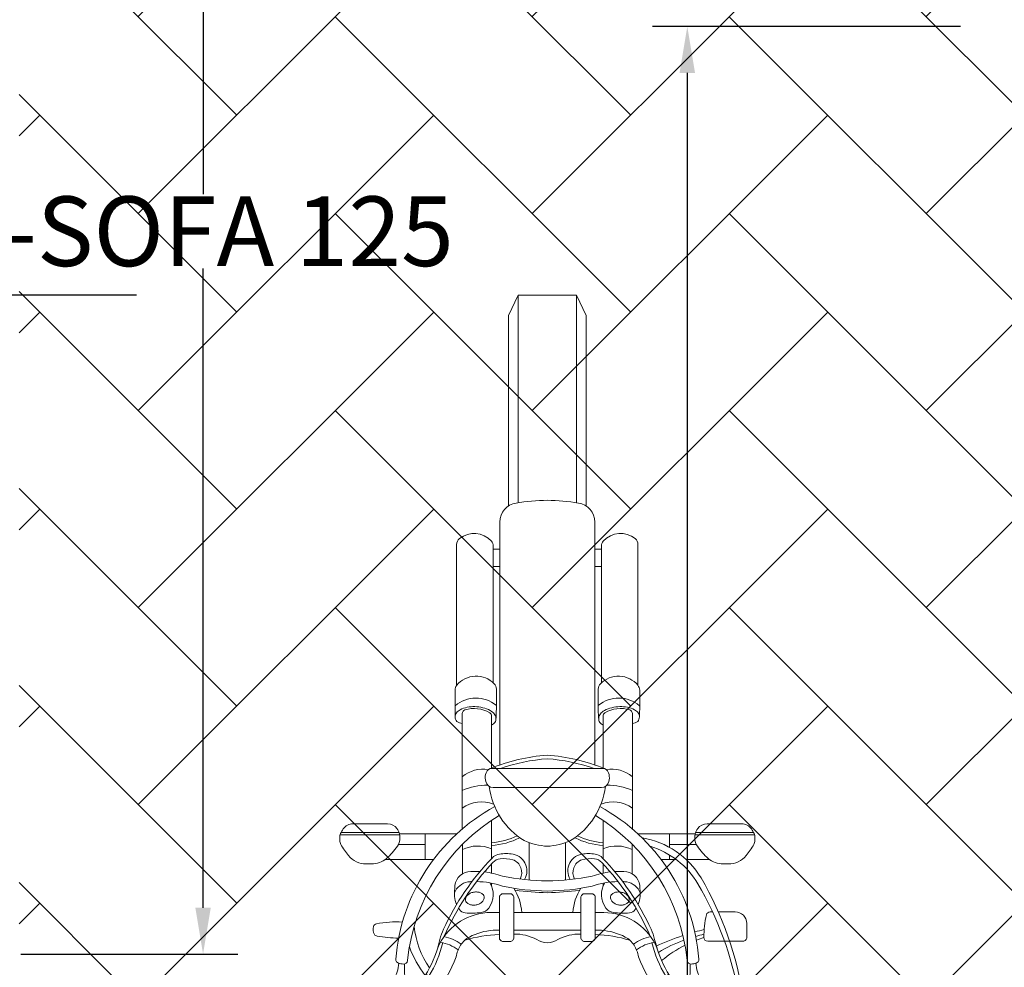
# Model space of a CAD drawing. Units: inches. Extents: x -466983 to 1020, y 324 to 318697.
# Tile 25 of 97: x 814 to 899, y 511 to 592. Entities that reach past the tile are written whole.
import ezdxf

# ---------------------------------------------------------------- set-up
doc = ezdxf.new("R2010")
doc.units = ezdxf.units.IN
doc.header["$MEASUREMENT"] = 0
for name, color, linetype, lineweight in [('A-ANNO-DIMS', 2, 'Continuous', 18), ('A-EQPM-VEHC', 8, 'Continuous', 18), ('A-FLOR-PATT', 252, 'Continuous', 13)]:
    doc.layers.add(name, color=color, linetype=linetype, lineweight=lineweight)
doc.styles.get("Standard").update_dxf_attribs({"font": 'arial.ttf'})
doc.dimstyles.get("Standard").update_dxf_attribs({"dimtxt": 6, "dimasz": 4, "dimexe": 3, "dimexo": 3, "dimgap": 0.09, "dimtad": 0, "dimtih": 1, "dimtoh": 1, "dimdec": 1, "dimzin": 0, "dimdsep": 46, "dimlunit": 3, "dimtxsty": 'Standard', "dimcen": 0.09, "dimadec": 0, "dimazin": 0, "dimtfac": 1, "dimtdec": 1, "dimtofl": 0, "dimtmove": 0, "dimatfit": 3, "dimfxl": 1, "dimtolj": 1, "dimtzin": 0, "dimarcsym": 0})

# ---------------------------------------------------------------- blocks, each defined once
blk = doc.blocks.new('Bike')
for p, q in [((3716.6, 1477), (3739.4, 1477)), ((3715.3, 1469.7), (3739.4, 1469.7)), ((3715, 1462.6), (3739.4, 1462.6)), ((3725.9, 1437.8), (3739.4, 1455.6)), ((3476.2, 1372.3), (3476.2, 1447.6)), ((3479.4, 1371.4), (3479.4, 1449.1)), ((3739.4, 1429.3), (3753.1, 1429.3)), ((4796.8, 1363.8), (4796.8, 1434.1)), ((3739.4, 1420.3), (3753.1, 1420.3)), ((3739.4, 1414.7), (3753.1, 1414.7)), ((3668.6, 1399.5), (3702.1, 1372.5)), ((3671.4, 1403.4), (3705.4, 1376.1)), ((3511.5, 1359.9), (3511.5, 1390.3)), ((4502.2, 1381), (4505.8, 1282.1)), ((3478.1, 1297.1), (3478.1, 1372)), ((3491.8, 1338.1), (3491.8, 1373.1)), ((4781.5, 1364.7), (4781.5, 1326.4)), ((3478.1, 1338.1), (3495.7, 1338.1)), ((3505.6, 1338.1), (3511.5, 1338.1)), ((3511.5, 1346.8), (3511.5, 1327.3)), ((4762.6, 1326.4), (4793.8, 1326.4)), ((4035.1, 1288.5), (4035.1, 1302.5)), ((3491.8, 1289.6), (3530.3, 1289.6)), ((4012.9, 1254.3), (4013.4, 1288.4)), ((4721.1, 1279.7), (4737.7, 1247.6)), ((4738.5, 1279.5), (4753.4, 1246.1)), ((3106.7, 1249.4), (3106.7, 1240.7)), ((3129.5, 1249.4), (3129.5, 1240.7)), ((3460.4, 1251.7), (3510.3, 1251.7)), ((3517.1, 1251.6), (3529.2, 1251.6)), ((3542.4, 1251.6), (3546.2, 1251.6)), ((4896.6, 1245.7), (4912.2, 1245.7)), ((3808.6, 1222.8), (3886.6, 1138)), ((3808.6, 1134.7), (3886.6, 1219.4)), ((3489.4, 1202.6), (3538.3, 1202.6)), ((3489.4, 1155.3), (3538.3, 1155.3)), ((3676.5, 1138.6), (3694.4, 1147.6)), ((3106.7, 1108.5), (3106.7, 1117.1)), ((3129.5, 1108.5), (3129.5, 1117.1)), ((3460.4, 1106.2), (3510.3, 1106.2)), ((3517.1, 1106.2), (3529.2, 1106.2)), ((3542.4, 1106.2), (3546.2, 1106.2)), ((4721.1, 1078.2), (4737.7, 1110.3)), ((4738.5, 1078.4), (4753.4, 1111.8)), ((4896.6, 1112.2), (4912.2, 1112.2)), ((4032.4, 1103.3), (4062.6, 1103.3)), ((4032.4, 1094.9), (4061.1, 1094.9)), ((3491.8, 1068.2), (3530.3, 1068.2)), ((4412.5, 1069.2), (4742.2, 1069.2)), ((3478.1, 1060.8), (3478.1, 985.9)), ((4461.5, 1046.8), (4489.1, 1046.8)), ((3511.5, 996.5), (3511.5, 1030.6)), ((4762.6, 1031.4), (4793.8, 1031.4)), ((4781.5, 993.1), (4781.5, 1031.4)), ((3478.1, 1019.8), (3500.2, 1019.8)), ((3491.8, 1019.8), (3491.8, 984.8)), ((3500.1, 1019.8), (3511.5, 1019.8)), ((3758.9, 1015.1), (3758.9, 983.2)), ((3758.9, 1002.4), (3851.5, 1002.4)), ((3511.5, 998), (3511.5, 967.6)), ((4796.8, 994.1), (4796.8, 923.8)), ((3476.2, 985.5), (3476.2, 910.3)), ((3479.4, 986.4), (3479.4, 908.8)), ((3668.6, 958.4), (3702.1, 985.4)), ((3671.4, 954.4), (3705.4, 981.8)), ((3739.4, 943.1), (3753.1, 943.1)), ((3739.4, 937.5), (3753.1, 937.5)), ((3739.4, 928.6), (3753.1, 928.6)), ((3725.9, 920.1), (3739.4, 902.3)), ((3755, 891.8), (3781.3, 909.1)), ((3715, 895.3), (3739.4, 895.3)), ((3715.3, 888.2), (3739.4, 888.2)), ((3716.6, 880.8), (3739.4, 880.8))]:
    blk.add_line(p, q)
for points in [[(3736.2, 1579.4), (3736.2, 1592.7, -0.414214), (3741.2, 1597.7), (3753.5, 1597.7, -0.414214), (3758.5, 1592.7), (3758.5, 1579.4, -0.414214), (3753.5, 1574.4), (3741.2, 1574.4, -0.414214)], [(3506.4, 1438.1, 0.044309), (3491.8, 1448.2, 0.12965), (3486.9, 1449.5), (3482.3, 1449.5, 0.116215), (3477.8, 1448.5, 0.026021), (3471.7, 1445, 0.256394), (3464.8, 1432.4), (3464.8, 1387.3, 0.252462), (3471.5, 1374.8, 0.012105), (3473, 1373.9, 0.288965), (3494.3, 1374.5, 0.06955), (3510.2, 1388.8, 0.177075), (3517.3, 1408.1), (3517.3, 1415, 0.223082)], [(4811.1, 1418.6, 0.390363), (4789.3, 1434.7, 0.055736), (4773.5, 1431.2, 0.196303), (4762.1, 1421.2, 0.154867), (4756.5, 1385.4, 0.215074), (4765.4, 1371.6, 0.140504), (4792.5, 1363.4, 0.387027), (4812.7, 1381.2, 0.07489)], [(3764.2, 1314.8, 0.116891), (3754.2, 1313.4, 0.104306), (3744.8, 1307.4, 0.090357), (3738.3, 1297.9, 0.08248), (3735, 1285.8, 0.08248), (3735.8, 1273.2, 0.090357), (3740.4, 1262.7, 0.104306), (3748.4, 1254.9, 0.116891), (3757.9, 1251.6, 0.116891), (3767.8, 1252.9, 0.104306), (3777.2, 1259, 0.090357), (3783.8, 1268.4, 0.08248), (3787.1, 1280.6, 0.08248), (3786.2, 1293.1, 0.090357), (3781.7, 1303.7, 0.104306), (3773.6, 1311.5, 0.116891)], [(4294.6, 1316.7, 0.093727), (4084.2, 1253.4, 0.26048), (4052.1, 1204.4, 0.011277), (4050.8, 1178.9, 0.011277), (4052.1, 1153.4, 0.26048), (4084.2, 1104.5, 0.093727), (4294.6, 1041.2, 0.168473), (4422.7, 1075.8, 0.123184), (4450.3, 1105.7, 0.12588), (4454, 1120.1), (4454, 1178.9), (4454, 1237.8, 0.12588), (4450.3, 1252.2, 0.123184), (4422.7, 1282.1, 0.168473)], [(3564.6, 1285.6, 0.137096), (3561.5, 1285.3, 0.107007), (3558.1, 1283.1, 0.081077), (3555.6, 1279.7, 0.06906), (3554.1, 1275, 0.06906), (3553.9, 1270, 0.081077), (3554.9, 1265.9, 0.107007), (3557.3, 1262.7, 0.137096), (3560.1, 1261.3, 0.137096), (3563.3, 1261.6, 0.107007), (3566.7, 1263.8, 0.081077), (3569.1, 1267.2, 0.06906), (3570.7, 1271.9, 0.06906), (3570.9, 1276.8, 0.081077), (3569.8, 1280.9, 0.107007), (3567.5, 1284.2, 0.137096)], [(3766.3, 1292.1, 0.136763), (3763.8, 1291.6, 0.10699), (3761.3, 1289.5, 0.081228), (3759.7, 1286.4, 0.069255), (3758.9, 1282.5, 0.069255), (3759.2, 1278.5, 0.081228), (3760.5, 1275.3, 0.10699), (3762.8, 1272.9, 0.136763), (3765.2, 1272.1, 0.136763), (3767.7, 1272.7, 0.10699), (3770.2, 1274.8, 0.081228), (3771.8, 1277.8, 0.069255), (3772.6, 1281.8, 0.069255), (3772.3, 1285.8, 0.081228), (3771, 1288.9, 0.10699), (3768.7, 1291.3, 0.136763)], [(3409.7, 1259.3, 0.088306), (3400.8, 1259.5, 0.265111), (3393, 1253.4, 0.077673), (3375.4, 1178.9, 0.077673), (3393, 1104.4, 0.265111), (3400.8, 1098.3, 0.088306), (3409.7, 1098.6, 0.355135), (3417.6, 1108.4), (3417.6, 1178.9), (3417.6, 1249.5, 0.355135)], [(4687.9, 1178.9, 0.027846), (4690.9, 1140.7, 0.357798), (4723.4, 1110.4, 0.096715), (4776.1, 1117.3, 0.32255), (4779.5, 1122.1), (4779.5, 1178.9), (4779.5, 1235.8, 0.32255), (4776.1, 1240.6, 0.096715), (4723.4, 1247.4, 0.357798), (4690.9, 1217.2, 0.027846)], [(3556.1, 1227.7), (3556.1, 1236.5, -0.414214), (3561.1, 1241.5), (3613.3, 1241.5, -0.414214), (3618.3, 1236.5), (3618.3, 1227.7, -0.414214), (3613.3, 1222.7), (3561.1, 1222.7, -0.414214)], [(3779.6, 1236, 0.198787), (3764.7, 1239.7, 0.033352), (3679.3, 1221.3, 0.334742), (3675.6, 1216.5), (3675.6, 1178.9), (3675.6, 1141.3, 0.334742), (3679.3, 1136.5, 0.033352), (3764.7, 1118.1, 0.198787), (3779.6, 1121.9, 0.220896), (3810.5, 1178.9, 0.220896)], [(4790.8, 1178.9), (4790.8, 1160.8, -0.145244), (4788.4, 1152.6, 0.168226), (4784.2, 1135.8, 0.389485), (4799.2, 1122.2, 0.058321), (4883.9, 1132.5, 0.346221), (4895.4, 1147.1), (4895.4, 1178.9), (4895.4, 1210.8, 0.346221), (4883.9, 1225.4, 0.058321), (4799.2, 1235.7, 0.389485), (4784.2, 1222, 0.168226), (4788.4, 1205.3, -0.145244), (4790.8, 1197.1)], [(3730.6, 1178.9, 0.074545), (3733.2, 1161.5, 0.085152), (3740.2, 1147.8, 0.106245), (3751.3, 1138, 0.128192), (3763.2, 1134.9, 0.128192), (3775.2, 1138, 0.106245), (3786.3, 1147.8, 0.085152), (3793.3, 1161.5, 0.074545), (3795.9, 1178.9, 0.074545), (3793.3, 1196.3, 0.085152), (3786.3, 1210.1, 0.106245), (3775.2, 1219.9, 0.128192), (3763.2, 1223, 0.128192), (3751.3, 1219.9, 0.106245), (3740.2, 1210.1, 0.085152), (3733.2, 1196.3, 0.074545)], [(3736.5, 1178.9, 0.070978), (3738.7, 1163.7, 0.082547), (3744.4, 1151.7, 0.106804), (3753.7, 1143.1, 0.13387), (3763.6, 1140.5, 0.13387), (3773.4, 1143.1, 0.106804), (3782.7, 1151.7, 0.082547), (3788.4, 1163.7, 0.070978), (3790.6, 1178.9, 0.070978), (3788.4, 1194.2, 0.082547), (3782.7, 1206.1, 0.106804), (3773.4, 1214.7, 0.13387), (3763.6, 1217.4, 0.13387), (3753.7, 1214.7, 0.106804), (3744.4, 1206.1, 0.082547), (3738.7, 1194.2, 0.070978)], [(3705.3, 1202.8, 0.162281), (3704.1, 1202.4, 0.10607), (3702.8, 1200.9, 0.070038), (3702.1, 1199, 0.056281), (3701.8, 1196.5, 0.056281), (3702.1, 1194, 0.070038), (3702.8, 1192.1, 0.10607), (3704.1, 1190.7, 0.162281), (3705.3, 1190.3, 0.162281), (3706.5, 1190.7, 0.10607), (3707.7, 1192.1, 0.070038), (3708.4, 1194, 0.056281), (3708.7, 1196.5, 0.056281), (3708.4, 1199, 0.070038), (3707.7, 1200.9, 0.10607), (3706.5, 1202.4, 0.162281)], [(3705.3, 1155.1, 0.162281), (3706.5, 1155.5, 0.10607), (3707.7, 1156.9, 0.070038), (3708.4, 1158.8, 0.056281), (3708.7, 1161.4, 0.056281), (3708.4, 1163.9, 0.070038), (3707.7, 1165.8, 0.10607), (3706.5, 1167.2, 0.162281), (3705.3, 1167.6, 0.162281), (3704.1, 1167.2, 0.10607), (3702.8, 1165.8, 0.070038), (3702.1, 1163.9, 0.056281), (3701.8, 1161.4, 0.056281), (3702.1, 1158.8, 0.070038), (3702.8, 1156.9, 0.10607), (3704.1, 1155.5, 0.162281)], [(3556.1, 1130.2), (3556.1, 1121.4, 0.414214), (3561.1, 1116.4), (3613.3, 1116.4, 0.414214), (3618.3, 1121.4), (3618.3, 1130.2, 0.414214), (3613.3, 1135.2), (3561.1, 1135.2, 0.414214)], [(3564.6, 1072.3, 0.137096), (3567.5, 1073.7, 0.107007), (3569.8, 1077, 0.081077), (3570.9, 1081, 0.06906), (3570.7, 1086, 0.06906), (3569.1, 1090.7, 0.081077), (3566.7, 1094.1, 0.107007), (3563.3, 1096.3, 0.137096), (3560.1, 1096.6, 0.137096), (3557.3, 1095.2, 0.107007), (3554.9, 1091.9, 0.081077), (3553.9, 1087.9, 0.06906), (3554.1, 1082.9, 0.06906), (3555.6, 1078.2, 0.081077), (3558.1, 1074.8, 0.107007), (3561.5, 1072.6, 0.137096)], [(4291, 1019.6), (4291, 1020, -0.414214), (4296, 1025), (4331.3, 1025, -0.414214), (4336.3, 1020), (4336.3, 1019.6, -0.414214), (4331.3, 1014.6), (4296, 1014.6, -0.414214)], [(3734.1, 992.8), (3734.1, 999.9, -0.414214), (3737.1, 1002.9), (3749.4, 1002.9, -0.414214), (3752.4, 999.9), (3752.4, 992.8, -0.414214), (3749.4, 989.8), (3737.1, 989.8, -0.414214)], [(4812.7, 976.7, 0.387027), (4792.5, 994.5, 0.140504), (4765.4, 986.3, 0.215074), (4756.5, 972.5, 0.154867), (4762.1, 936.7, 0.196303), (4773.5, 926.7, 0.055736), (4789.3, 923.2, 0.390363), (4811.1, 939.2, 0.07489)], [(3517.3, 942.8), (3517.3, 949.8, 0.177075), (3510.2, 969.1, 0.06955), (3494.3, 983.4, 0.288965), (3473, 984, 0.012105), (3471.5, 983.1, 0.252462), (3464.8, 970.6), (3464.8, 925.5, 0.256394), (3471.7, 912.9, 0.026021), (3477.8, 909.4, 0.116215), (3482.3, 908.4), (3486.9, 908.4, 0.12965), (3491.8, 909.7, 0.044309), (3506.4, 919.8, 0.223082)], [(3780.1, 689), (3790, 689, 0.414214), (3791, 690), (3791, 832.2, 0.414214), (3790, 833.2), (3780.1, 833.2, 0.414214), (3779.1, 832.2), (3779.1, 690, 0.414214)], [(3736.2, 778.4), (3736.2, 765.2, 0.414214), (3741.2, 760.2), (3753.5, 760.2, 0.414214), (3758.5, 765.2), (3758.5, 778.4, 0.414214), (3753.5, 783.4), (3741.2, 783.4, 0.414214)]]:
    blk.add_lwpolyline(points, format="xyb", close=True)
for points in [[(3713.9, 1447.6, 0.022793), (3715.3, 1473.8, 0.136), (3726.4, 1569.3)], [(3739.4, 1574.8), (3739.4, 1409.9, 0.414214), (3744.4, 1404.9), (3748.1, 1404.9, 0.414214), (3753.1, 1409.9), (3753.1, 1574.4)], [(3691, 1434, -0.079005), (3686.9, 1465, -0.05973), (3703.5, 1491.3, 0.159047), (3718.1, 1528.9, 0.126021), (3710.9, 1564.4)], [(3753.1, 1463), (3798.3, 1533.8, -0.40834), (3811.9, 1536.9), (3824.4, 1529.3, -0.431541), (3827.4, 1515.1), (3781.3, 1448.7), (3755, 1466.1)], [(3779.1, 1525.7, 0.414214), (3780.1, 1524.7), (3790, 1524.7, 0.414214), (3791, 1525.7)], [(3742, 1424.6), (3692.9, 1464.8, 0.483058), (3685.2, 1463.1, 0.088789), (3676.2, 1431.5)], [(3579.8, 1394.4), (3579.8, 1391.2, 0.349421), (3583.7, 1386.3, 0.057073), (3613.1, 1383, 0.413662), (3618.1, 1388), (3618.1, 1433.9, 0.414214), (3613.1, 1438.9), (3594.8, 1438.9, 0.414214), (3579.8, 1423.9), (3579.8, 1401.9)], [(3737.5, 1420.6), (3706.2, 1444.8, 0.431039), (3699, 1443.7), (3669.3, 1400.5, 0.337774), (3670.5, 1376.2, 0.230362), (3695.1, 1365.4)], [(3741.3, 1406, -0.159938), (3748.2, 1383.3, 0.280919), (3781.3, 1448.7)], [(3692.5, 1434.2, 0.096183), (3535.6, 1379.4, 0.22037), (3483.3, 1302.5)], [(3688.4, 1428.2, 0.089404), (3543.1, 1375.3, 0.184983), (3494.2, 1313)], [(3537.7, 1208.8, -0.564837), (3504.3, 1226.3, -0.102735), (3505.1, 1243.5, -0.140154), (3509.2, 1250.6, -0.082892), (3602.5, 1314.4, -0.053437), (3615.6, 1318.8, 0.151196), (3693.3, 1363.4, 0.070423), (3739.4, 1423.8)], [(3603.7, 1241.5), (3603.7, 1249.5, -0.101252), (3612.6, 1280.5, -0.13244), (3623.3, 1292, -0.090169), (3638.2, 1297.9, 0.164837), (3725.3, 1368), (3729.9, 1373.3, 0.174158), (3734.8, 1386, 0.159727), (3728.6, 1406.2)], [(3454.1, 1241.7, -0.235435), (3643.3, 1361.2, 0.410863), (3647.8, 1366.7, 0.044254), (3646.7, 1372.8, 0.360214), (3641.5, 1376.5, 0.253572), (3442.6, 1247.5)], [(4589, 1290), (4585.2, 1365.1, 0.35984), (4576.7, 1374.5, 0.038725), (4466.4, 1381.4, 0.009033), (4191, 1365, 0.303597), (4182.3, 1358.1, 0.12706), (4178.4, 1294.5)], [(4421.3, 1283), (4757.5, 1279.3, 0.417467), (4762.6, 1284.3), (4762.6, 1373.6)], [(3864.3, 1338.9, 0.080734), (3852.8, 1356, 0.212509), (3837.8, 1362.2, 0.038096), (3711.9, 1349.7)], [(3851.8, 1356.9, 0.001252), (4028.5, 1349.8, 0.046276), (4039.5, 1350.4, 0.000101), (4174.5, 1370.4, -0.314799), (4184.8, 1365.3), (4186, 1363.2)], [(4746.4, 1261.7), (4788.8, 1261.7, 0.414214), (4793.8, 1266.7), (4793.8, 1363.4)], [(3711.6, 1008.5, 0.070303), (3742.4, 1010.7, 0.039628), (4030.9, 1111.4, 0.282444), (4048.7, 1137.2, 0.015247), (4049.8, 1178.9, 0.015247), (4048.7, 1220.7, 0.282444), (4030.9, 1246.5, 0.039628), (3742.4, 1347.2, 0.070303), (3711.6, 1349.4)], [(4004.7, 1257.8, 0.018709), (4004.5, 1312.9, 0.375923), (3986.3, 1332, 0.029426), (3773.7, 1338.7)], [(4301, 1317, -0.138428), (4310.6, 1341, -0.233155), (4318.5, 1344.9), (4374.8, 1344.9, -0.216687), (4382.4, 1341.5, -0.156826), (4390.4, 1322.8)], [(4354.1, 1312.1, 0.056144), (4350.9, 1321, 0.085082), (4347.3, 1326.2, 0.153535), (4342.4, 1328.6, 0.197677), (4338.3, 1327.7, 0.1268), (4335.1, 1324, 0.072333), (4332.4, 1315.8, 0.051836)], [(4479.1, 1282.4, 0.326046), (4467.3, 1323.7, 0.2025), (4459.8, 1325.7, -0.079204), (4344.5, 1328.2)], [(3611.5, 1313.2, 0.084453), (3515.3, 1250, 0.185223), (3510.6, 1240.3, 0.080228), (3511.8, 1223.9, 0.449113), (3537, 1214.3)], [(3627.1, 1321.9, 0.043315), (3622.3, 1319.9, 0.279952), (3580.6, 1252.4), (3580.6, 1241.5)], [(3757.9, 1314.5, 0.058653), (3749, 1313.6, 0.314496), (3730.4, 1291.7, 0.11242), (3732.3, 1267.9, 0.161441), (3739.7, 1257.7, 0.088312), (3749.1, 1253.2, 0.094137), (3758.6, 1251.5)], [(3284.5, 1297.1), (3100.9, 1297.1, 0.226605), (3093.1, 1293.4, 0.400758), (3096.5, 1251.9, 0.183413), (3103.2, 1249.4), (3281.2, 1249.4)], [(3324.7, 1299.2, 0.006041), (3316.2, 1299.3), (3290.7, 1299.3, 0.172401), (3284.4, 1297, 0.450807), (3282.4, 1248.2, 0.193514), (3289.3, 1245.4), (3311, 1245.4, 0.017498), (3327.2, 1245.7)], [(3334.2, 1289.8, 0.161741), (3331.4, 1296.9, 0.157572), (3325.7, 1299, 0.171418), (3320.4, 1297.4, 0.113331), (3316.3, 1292.6, 0.072079), (3313, 1283.4, 0.055689), (3312.2, 1273.3, 0.053775), (3313.6, 1263, 0.064911), (3317.3, 1253.4, 0.09694), (3321.7, 1248.1, 0.155824), (3327.4, 1245.9, 0.172526), (3332.7, 1247.4, 0.151352), (3336.2, 1251.6)], [(3570.1, 1297.2, 0.144644), (3549.1, 1299.6, 0.369621), (3527.5, 1282.5, 0.036315), (3527.3, 1266.8)], [(3555, 1300.1, 0.253732), (3540.7, 1282.5, 0.012512), (3540.3, 1277.1)], [(4050.2, 1288.6, 0.000873), (4050.2, 1288.7, 0.265813), (4035.8, 1302.3, 0.056152), (4004.7, 1306.3)], [(4481.3, 1293.5), (4486.7, 1293.8, 0.420229), (4488.6, 1296), (4488.1, 1302.3, 0.415516), (4485.9, 1304.1), (4480.3, 1303.7)], [(3392.3, 1251.6), (3324.6, 1251.6, -0.26356), (3320.3, 1254, -0.214715), (3316.5, 1286.3, -0.327171), (3321.3, 1289.8), (3471.6, 1289.8)], [(3541.9, 1253.9, 0.31484), (3574.9, 1255.4, 0.193965), (3580.6, 1265, 0.061634), (3581.2, 1286.2, 0.219833), (3576.9, 1293.4, 0.014528), (3575.1, 1294.6)], [(4005.1, 1288.4), (4101.4, 1288.7, -0.407202), (4111.4, 1279), (4111.7, 1266.7)], [(3540.3, 1086.8, -0.079272), (3546.2, 1120.5, 0.050281), (3552.6, 1178.9, 0.050281), (3546.2, 1237.4, -0.079272), (3540.3, 1271.1)], [(4721.2, 1103.2, 0.004418), (4491.2, 1094.2, -0.414214), (4481.2, 1084.2), (4474.7, 1084.2, -0.414214), (4464.7, 1094.2), (4464.7, 1178.9), (4464.7, 1263.7, -0.414214), (4474.7, 1273.7), (4481.2, 1273.7, -0.414214), (4491.2, 1263.7)], [(4720.8, 1279.7, 0.108929), (4717, 1269, 0.145286), (4718.3, 1260.6), (4724.6, 1247.5)], [(3527.8, 1096.9, -0.055925), (3533.1, 1120.5, 0.050281), (3539.5, 1178.9, 0.050281), (3533.1, 1237.4, -0.055925), (3527.8, 1261)], [(4491.2, 1094.2), (4491.2, 1178.9), (4491.2, 1263.7, 0.004418), (4721.2, 1254.7)], [(4705.9, 1241.5, 0.063368), (4580, 1258, -0.001705), (4491.2, 1262)], [(4926.4, 1206.2), (4926.4, 1264.5, 0.414214), (4921.4, 1269.5), (4917.2, 1269.5, 0.414214), (4912.2, 1264.5), (4912.2, 1210.4)], [(3416.3, 1103.3, 0.231711), (3486.9, 1148.9, 0.086055), (3494.3, 1178.9, 0.086055), (3486.9, 1209, 0.231711), (3416.3, 1254.6)], [(4736.9, 1247.6, 0.067766), (4724, 1178.9, 0.067766), (4736.9, 1110.2)], [(4748.9, 1102, 0.004183), (4881.9, 1107.1, 0.304225), (4904.8, 1123, 0.085326), (4916.2, 1178.9, 0.085326), (4904.8, 1234.8, 0.304225), (4881.9, 1250.8, 0.004183), (4748.9, 1255.9)], [(3388.2, 1117.1), (3071.5, 1117.1, -0.369002), (3046.8, 1138.2, -0.033307), (3043.1, 1178.9, -0.033307), (3046.8, 1219.6, -0.369002), (3071.5, 1240.7), (3388.2, 1240.7)], [(3392.7, 1239.9, 0.062968), (3380.1, 1178.9, 0.062968), (3392.7, 1118)], [(3694.4, 1210.2), (3694.4, 1178.9), (3694.4, 1147.6, 0.084607), (3762, 1124, 0.24184), (3783.8, 1130.9, 0.177565), (3806.3, 1178.9, 0.177565), (3783.8, 1227, 0.24184), (3762, 1233.9, 0.084607), (3694.4, 1210.2), (3676.5, 1219.3)], [(3551.4, 1136.8, 0.036141), (3554.8, 1178.9, 0.036141), (3551.4, 1221.1)], [(3608.7, 1135.2, -0.133909), (3615.9, 1165.1, 0.12166), (3620.2, 1178.9, 0.12166), (3615.9, 1192.7, -0.133909), (3608.7, 1222.7)], [(4913.1, 1206.2), (4940.3, 1206.2, -0.414214), (4955.3, 1191.2), (4955.3, 1178.9), (4955.3, 1166.7, -0.414214), (4940.3, 1151.7), (4913.1, 1151.7)], [(3537.7, 1149.1, 0.564837), (3504.3, 1131.6, 0.102735), (3505.1, 1114.4, 0.140154), (3509.2, 1107.3, 0.082892), (3602.5, 1043.5, 0.053437), (3615.6, 1039, -0.151196), (3693.3, 994.4, -0.070423), (3739.4, 934)], [(3537, 1143.6, 0.449113), (3511.8, 1134, 0.080228), (3510.6, 1117.6, 0.185223), (3515.3, 1107.9, 0.084453), (3611.5, 1044.6)], [(4912.2, 1147.5), (4912.2, 1093.4, 0.414214), (4917.2, 1088.4), (4921.4, 1088.4, 0.414214), (4926.4, 1093.4), (4926.4, 1151.7)], [(3281.2, 1108.5), (3103.2, 1108.5, 0.183413), (3096.5, 1106, 0.400758), (3093.1, 1064.5, 0.226605), (3100.9, 1060.7), (3284.5, 1060.7)], [(3327.2, 1112.1, 0.017498), (3311, 1112.5), (3289.3, 1112.5, 0.193514), (3282.4, 1109.7, 0.450807), (3284.4, 1060.8, 0.172401), (3290.7, 1058.6), (3316.2, 1058.6, 0.006041), (3324.7, 1058.7)], [(3336.2, 1106.3, 0.151352), (3332.7, 1110.5, 0.172526), (3327.4, 1112, 0.155824), (3321.7, 1109.8, 0.09694), (3317.3, 1104.4, 0.064911), (3313.6, 1094.9, 0.053775), (3312.2, 1084.5, 0.055689), (3313, 1074.5, 0.072079), (3316.3, 1065.2, 0.113331), (3320.4, 1060.5, 0.171418), (3325.7, 1058.8, 0.157572), (3331.4, 1060.9, 0.161741), (3334.2, 1068.1)], [(3392.3, 1106.3), (3324.6, 1106.3, 0.26356), (3320.3, 1103.8, 0.214715), (3316.5, 1071.6, 0.327171), (3321.3, 1068.1), (3471.6, 1068.1)], [(3442.6, 1110.3, 0.253572), (3641.5, 981.4, 0.360214), (3646.7, 985.1, 0.044254), (3647.8, 991.2, 0.410863), (3643.3, 996.6, -0.235435), (3454.1, 1116.2)], [(3575.1, 1063.2, 0.014528), (3576.9, 1064.4, 0.219833), (3581.2, 1071.7, 0.061634), (3580.6, 1092.8, 0.193965), (3574.9, 1102.5, 0.31484), (3541.9, 1104)], [(3580.6, 1116.4), (3580.6, 1105.5, 0.279952), (3622.3, 1037.9, 0.043315), (3627.1, 1036)], [(3728.6, 951.6, 0.159727), (3734.8, 971.9, 0.174158), (3729.9, 984.5), (3725.3, 989.8, 0.164837), (3638.2, 1059.9, -0.090169), (3623.3, 1065.9, -0.13244), (3612.6, 1077.3, -0.101252), (3603.7, 1108.3), (3603.7, 1116.4)], [(4032.4, 1112), (4032.4, 1054.3, -0.140419), (4030.9, 1049), (4028.4, 1045)], [(4069.3, 1115.5, 0.182977), (4061, 1091.7, 0.292151), (4070, 1078.3, 0.060635), (4155.6, 1053.1)], [(4491.2, 1095.9, -0.001705), (4580, 1099.9, 0.063368), (4705.9, 1116.4)], [(4724.6, 1110.4), (4718.3, 1097.3, 0.145286), (4717, 1088.8, 0.108929), (4720.8, 1078.2)], [(3527.3, 1091.1, 0.036315), (3527.5, 1075.3, 0.369621), (3549.1, 1058.3, 0.144644), (3570.1, 1060.7)], [(4793.8, 994.5), (4793.8, 1091.2, 0.414214), (4788.8, 1096.2), (4746.4, 1096.2)], [(3540.3, 1080.8, 0.012512), (3540.7, 1075.3, 0.253732), (3555, 1057.8)], [(4379.8, 1053.5), (4735.9, 1053.5, 0.378085), (4740.8, 1057.9), (4743.4, 1078.4)], [(4762.6, 984.3), (4762.6, 1073.6, 0.417467), (4757.5, 1078.6), (4421.3, 1074.8)], [(3860.2, 1000.8), (3860.2, 1006.9, -0.339938), (3867.7, 1016.5, 0.159134), (3905.8, 1041.3, -0.226589), (3913.5, 1045), (4055.5, 1045, 0.174252), (4068.2, 1049.6), (4069.7, 1050.8, -0.174252), (4076, 1053.1), (4223.9, 1053.1)], [(4338.2, 993.7, -0.040508), (4365, 997.7, -0.03842), (4428.6, 995.4, 0.607774), (4471.6, 1015.9), (4471.5, 1027, 0.485016), (4437.8, 1051.6, -0.00298), (4362, 1047.8)], [(4485.9, 1020.1, 0.170118), (4536.9, 1031.7, 0.477675), (4537.8, 1039.4, 0.09469), (4517.6, 1053.5)], [(4316, 1014.6, 0.114491), (4321.5, 997.6, 0.239101), (4329.2, 992.8, 0.103983), (4339, 994, 0.167173), (4344.1, 997.9, 0.363558), (4338.9, 1042.9)], [(4532, 1028.9), (4637, 1028.9, 0.414214), (4642, 1033.9), (4642, 1037.6, 0.414214), (4637, 1042.6), (4534.5, 1042.6)], [(4470.4, 1033.9), (4480.9, 1033.9, -0.414214), (4485.9, 1028.9), (4485.9, 1008.2, -0.414214), (4480.9, 1003.2), (4467.9, 1003.2)], [(3741.8, 978.4, 0.005304), (3743.1, 983.2), (3959.4, 983.2, -0.102096), (3963.4, 982.4, 0.00244), (3995.8, 968.6, 0.501027), (4009.6, 976.7, 0.054221), (4009.7, 990, 0.228934), (4005.1, 997.3, 0.079407), (3985, 1006, 0.239312), (3976.1, 1004, -0.075874), (3957.8, 993, -0.0999), (3953.9, 992.2, -0.077513), (3779.8, 1020.9)], [(4296.5, 1014.6, 0.031683), (4298.6, 996.5, 0.319342), (4310.9, 984.3, 0.078645), (4373.6, 984.1, 0.339222), (4377.8, 988.5, 0.096684), (4377, 998)], [(3593, 990.1, 0.064082), (3595.5, 956.1, 0.274699), (3598.9, 952.4, 0.213807), (3609.1, 953.6, 0.217468), (3611.4, 957.1, 0.038755), (3614, 985.1)], [(3695.1, 992.5, 0.230362), (3670.5, 981.6, 0.337774), (3669.3, 957.4), (3699, 914.2, 0.431039), (3706.2, 913.1), (3737.5, 937.3)], [(3753.1, 894.9), (3798.3, 824.1, 0.40834), (3811.9, 820.9), (3824.4, 828.5, 0.431541), (3827.4, 842.8), (3781.3, 909.1, 0.280919), (3748.2, 974.6, -0.159938), (3741.3, 951.9)], [(3753.1, 783.4), (3753.1, 948, 0.414214), (3748.1, 953), (3744.4, 953, 0.414214), (3739.4, 948), (3739.4, 783.1)], [(3676.4, 947.1, 0.047742), (3675.9, 929.4), (3675.9, 929.3, 0.096803), (3685.2, 894.8, 0.483058), (3692.9, 893.1), (3742, 933.3)], [(3691.4, 925.3, 0.082553), (3686.9, 892.9, 0.05973), (3703.5, 866.6, -0.159047), (3718.1, 829, -0.126021), (3710.9, 793.5)], [(3726.4, 788.6, 0.136), (3715.3, 884.1, 0.022793), (3713.9, 910.3)]]:
    blk.add_lwpolyline(points, format="xyb")
for points in [[(4537.3, 1281.8), (4545.1, 1290), (4630.1, 1290), (4643.2, 1280.6)], [(3392.7, 1105.3), (3392.7, 1178.9), (3392.7, 1252.6)], [(4831, 1234.2), (4831, 1178.9), (4831, 1123.7)], [(3050.6, 1229.4), (2939.7, 1229.4), (2802.2, 1229.4), (2775.9, 1217), (2775.9, 1164.4)], [(3580.6, 1222.7), (3580.6, 1178.9), (3580.6, 1135.2)], [(3603.7, 1222.7), (3603.7, 1178.9), (3603.7, 1135.2)], [(2776, 1217), (2957.8, 1217), (3046.4, 1217)], [(3050.6, 1128.5), (2939.7, 1128.5), (2802.2, 1128.5), (2775.9, 1140.9), (2775.9, 1193.5)], [(2776, 1140.9), (2957.8, 1140.9), (3046.4, 1140.9)]]:
    blk.add_lwpolyline(points)
for centre, radius in [((3716.6, 1573.3), 10.6), ((3845.9, 1178.7), 57.6), ((3716.6, 784.6), 10.6)]:
    blk.add_circle(centre, radius)
for centre, radius, start, end in [((3741.5, 1637.1), 41.2, 286.9888, 312.0372), ((3749, 1534.6), 40.1, 57.3492, 83.449), ((3788.9, 1493.4), 40.9, 27.2359, 77.1495), ((3769, 1422), 93.3, 177.6075, 186.9102), ((3908.5, 1569.9), 206.8, 221.2614, 229.5793), ((3710.3, 1384.2), 37.9, 39.0272, 51.9723), ((3680.5, 1359.4), 91.4, 24.0671, 37.4396), ((3939.5, 1465.4), 346.6, 193.685, 195.7923), ((3803.7, 1426.1), 199.4, 192.4698, 195.6556), ((3774.2, 1434.7), 169, 197.8118, 201.3124), ((3639.5, 1433), 61.1, 276.8609, 298.2339), ((3711.2, 1436.9), 65.1, 287.813, 304.5915), ((3515.3, 1317.4), 234.8, 9.2486, 15.3175), ((3649, 1152.2), 213.1, 78.6059, 90.3415), ((3597.6, 1291.6), 626.2, 1.209, 6.9337), ((3939.5, 1465.4), 346.6, 198.4449, 204.6334), ((3803.7, 1426.1), 199.4, 200.2574, 210.9013), ((3774.2, 1434.7), 169, 206.8349, 219.1999), ((3923.3, 1335), 33.4, 359.0902, 32.2964), ((3841.7, 1313.3), 185.9, 357.1486, 11.3635), ((3834.7, 1458.1), 211.7, 214.8443, 221.5826), ((3842.4, 1463.3), 211.7, 214.9067, 221.5218), ((3733.5, 1322.4), 116.7, 356.6367, 8.2567), ((4387.6, 1310.4), 62.2, 146.2979, 174.4306), ((4408.7, 1315.7), 68.7, 154.8594, 169.0097), ((4355, 1321.8), 28.2, 18.3548, 54.9232), ((3584.9, 1462.7), 151.5, 283.3715, 301.3249), ((4337, 1290.1), 53.6, 11.0089, 38.6482), ((4349.2, 1289.8), 53.6, 4.6068, 37.9011), ((4362.7, 1290.1), 53.6, 356.0108, 36.9065), ((4374.9, 1290.1), 53.6, 352.3592, 36.9849), ((4386.5, 1290.4), 53.6, 351.8913, 37.1496), ((4388.7, 1287), 62.9, 356.0657, 35.4453), ((4364.1, 1281), 94.8, 0.9619, 27.161), ((3664.1, 1323.1), 52.9, 190.2344, 217.1371), ((3671.6, 1327), 52.9, 189.3206, 216.9338), ((3343.1, 1272.2), 42, 139.9272, 219.6749), ((3435.7, 1263), 41.9, 140.3451, 189.8858), ((3483.9, 1259.5), 69.2, 154.0504, 182.4153), ((3479.7, 1264.6), 43.4, 144.5037, 201.1055), ((3538.9, 1269.4), 45, 153.363, 203.2549), ((3783.3, 1235.1), 174.2, 162.8434, 177.8981), ((4165.8, 1215.8), 79.7, 77.8259, 132.9545), ((4481.9, 1161.8), 112.1, 93.7127, 111.5258), ((3394.4, 1259.4), 95.6, 334.4456, 355.3484), ((3397.9, 1258.1), 95.6, 333.0513, 356.1505), ((3585.6, 1280.9), 68.9, 237.8956, 265.8204), ((3397.9, 1099.8), 95.6, 3.8495, 26.9487), ((3585.6, 1077), 68.9, 94.1796, 122.1044), ((3394.4, 1098.5), 95.6, 4.6516, 25.5544), ((3343.1, 1085.7), 42, 140.3251, 220.0728), ((3479.7, 1093.3), 43.4, 158.8945, 215.4963), ((3538.9, 1088.4), 45, 156.7451, 206.637), ((3783.3, 1122.7), 174.2, 182.1019, 197.1566), ((3435.7, 1094.9), 41.9, 170.1142, 219.6549), ((3483.9, 1098.4), 69.2, 177.5847, 205.9496), ((4481.9, 1196.1), 112.1, 248.4742, 266.2873), ((3664.1, 1034.8), 52.9, 142.8629, 169.7656), ((4027.2, 1133.1), 111.1, 213.3859, 232.4739), ((3671.6, 1030.9), 52.9, 143.0662, 170.6794), ((4082.7, 908.2), 205.4, 132.3055, 138.2462), ((4528.9, 1021.1), 47.3, 136.8041, 165.0837), ((3584.9, 895.2), 151.5, 58.6751, 76.6285), ((3834.7, 899.8), 211.7, 138.4174, 145.1557), ((4440.3, 1021.4), 143.9, 172.1779, 178.584), ((4355.4, 1018.1), 39.6, 144.2076, 169.9356), ((4336.5, 1017), 40.3, 331.7508, 49.9014), ((4349.2, 1019.2), 42.2, 329.8767, 44.2278), ((4363.9, 1017.8), 42.2, 331.3167, 48.0597), ((4376.7, 1015.8), 42.2, 333.1337, 53.4177), ((4391.4, 1013.8), 42.2, 333.4944, 59.7642), ((4402.5, 1013.1), 42.2, 327.9971, 63.0183), ((3842.4, 894.6), 211.7, 138.4782, 145.0933), ((3586.6, 1121.8), 117.1, 275.9386, 304.5183), ((3566.8, 1150.4), 162.3, 291.2356, 306.3114), ((3649, 1205.7), 213.1, 269.6585, 281.3941), ((3639.5, 924.8), 61.1, 61.7661, 83.1391), ((3711.2, 921), 65.1, 55.4085, 72.187), ((3680.5, 998.5), 91.4, 322.5604, 335.9329), ((3710.3, 973.7), 37.9, 308.0277, 320.9728), ((3908.5, 788), 206.8, 130.4207, 138.7386), ((3788.9, 864.5), 40.9, 282.8505, 332.7641), ((4007, 761.1), 238.1, 163.1793, 196.8207), ((3749, 823.3), 40.1, 276.551, 302.6508), ((3741.5, 720.8), 41.2, 47.9628, 73.0112)]:
    blk.add_arc(centre, radius, start, end)
blk = doc.blocks.new('*D69')
at = {"layer": 'A-ANNO-DIMS', "color": 0, "lineweight": -2, "transparency": 16777216}
for p, q in [((813.968, 636.229), (832.65, 636.229)), ((829.65, 632.229), (829.65, 577.152)), ((829.65, 515.686), (829.65, 570.763)), ((813.968, 511.686), (832.65, 511.686))]:
    blk.add_line(p, q, dxfattribs=at)
at = {"layer": 'A-ANNO-DIMS', "color": 0, "transparency": 16777216}
for points in [[(828.983, 632.229), (830.316, 632.229), (829.65, 636.229)], [(828.983, 515.686), (830.316, 515.686), (829.65, 511.686)]]:
    blk.add_solid(points, dxfattribs=at)
at = {"layer": 'Defpoints', "color": 0, "transparency": 16777216}
for p in [(810.968, 636.229), (829.65, 636.229), (810.968, 511.686)]:
    blk.add_point(p, dxfattribs=at)
at = {"layer": 'A-ANNO-DIMS', "color": 0, "transparency": 16777216, "insert": (829.65, 573.958), "char_height": 6, "attachment_point": 5}
blk.add_mtext('\\A1;L-SOFA 125', dxfattribs=at)
blk = doc.blocks.new('*D95')
at = {"layer": 'A-ANNO-DIMS', "color": 0, "lineweight": -2, "transparency": 16777216}
for p, q in [((894.884, 591.598), (868.36, 591.598)), ((871.36, 587.598), (871.36, 506.376)), ((871.36, 418.769), (871.36, 499.991)), ((894.884, 414.769), (868.36, 414.769))]:
    blk.add_line(p, q, dxfattribs=at)
at = {"layer": 'A-ANNO-DIMS', "color": 0, "transparency": 16777216}
for points in [[(870.693, 587.598), (872.026, 587.598), (871.36, 591.598)], [(870.693, 418.769), (872.026, 418.769), (871.36, 414.769)]]:
    blk.add_solid(points, dxfattribs=at)
at = {"layer": 'Defpoints', "color": 0, "transparency": 16777216}
for p in [(897.884, 591.598), (871.36, 414.769), (897.884, 414.769)]:
    blk.add_point(p, dxfattribs=at)
at = {"layer": 'A-ANNO-DIMS', "color": 0, "transparency": 16777216, "insert": (871.36, 503.184), "char_height": 6, "attachment_point": 5}
blk.add_mtext('\\A1;CAR 177', dxfattribs=at)
blk = doc.blocks.new('*D97')
at = {"layer": 'A-ANNO-DIMS', "color": 0, "lineweight": -2, "transparency": 16777216}
for p, q in [((823.929, 568.441), (802.329, 568.441)), ((805.329, 564.441), (805.329, 499.545)), ((805.329, 428.441), (805.329, 493.337)), ((823.929, 424.441), (802.329, 424.441))]:
    blk.add_line(p, q, dxfattribs=at)
at = {"layer": 'A-ANNO-DIMS', "color": 0, "transparency": 16777216}
for points in [[(804.662, 564.441), (805.996, 564.441), (805.329, 568.441)], [(804.662, 428.441), (805.996, 428.441), (805.329, 424.441)]]:
    blk.add_solid(points, dxfattribs=at)
at = {"layer": 'Defpoints', "color": 0, "transparency": 16777216}
for p in [(826.929, 568.441), (805.329, 424.441), (826.929, 424.441)]:
    blk.add_point(p, dxfattribs=at)
at = {"layer": 'A-ANNO-DIMS', "color": 0, "transparency": 16777216, "insert": (805.329, 496.441), "char_height": 6, "attachment_point": 5}
blk.add_mtext('\\A1;BIKE 144', dxfattribs=at)

msp = doc.modelspace()

# ---------------------------------------------------------------- hatches: boundary and pattern name
at = {"layer": 'A-FLOR-PATT', "transparency": 33554572}
h = msp.add_hatch(dxfattribs=at)
h.set_pattern_fill('ANSI37', color=256, scale=30)
h.set_pattern_definition([(45, (-1212.4137, -290.035), (-2.6516504, 2.6516504), []), (135, (-1212.4137, -290.035), (-2.6516504, -2.6516504), [])])
h.paths.add_polyline_path([(901.806, 1075.938), (900.614, 1075.938), (900.614, 1065.386), (899.391, 1065.386), (898.091, 1065.386), (892.836, 1058.71, -0.258377), (892.188, 1058.351), (879.985, 1058.351, -0.20177), (879.438, 1058.581), (874.081, 1065.386), (872.781, 1065.386), (871.558, 1065.386), (871.558, 1075.938), (813.806, 1075.938), (813.806, 1044.792), (832.395, 1044.792, -0.394795), (848.66, 1028.536), (848.66, 1009.938), (901.806, 1009.938), (901.806, 1015.938), (901.306, 1015.938), (871.306, 1015.938), (871.306, 1017.25), (871.334, 1017.25, -0.401453), (901.306, 1045.938), (901.806, 1045.938)])
edge = h.paths.add_edge_path(flags=16)
edge.add_line((847.773, 1068.949), (847.773, 1073.709))
edge.add_arc((849.227, 1073.709), 1.454, 90, 180, ccw=False)
edge.add_line((849.227, 1075.163), (864.492, 1075.163))
edge.add_arc((864.492, 1073.709), 1.454, 0, 90, ccw=False)
edge.add_line((865.946, 1073.709), (865.946, 1069.004))
edge.add_arc((832.645, 1068.976), 33.301, -20.61234, 0.04725, ccw=False)
edge.add_ellipse((856.859, 1058.48), major_axis=(0, 10.213), ratio=0.685919, start_angle=100.00884, end_angle=259.99116, ccw=False)
edge.add_arc((881.074, 1068.976), 33.301, 180.04725, 200.61234, ccw=False)
h.paths.add_polyline_path([(853.146, 1066.482), (853.146, 1066.453), (853.146, 1066.453, 0.433107), (852.917, 1066.685), (852.917, 1066.453), (853.146, 1066.453), (853.146, 1066.482), (853.088, 1066.612, 0.697939), (852.7, 1066.453), (852.7, 1066.453), (852.7, 1066.482), (852.917, 1067.001), (852.917, 1066.685, -0.396254)], flags=0)
h.paths.add_polyline_path([(861.019, 1066.482), (861.019, 1066.453), (861.019, 1066.453, 0.416404), (860.802, 1066.685), (860.802, 1066.453), (861.019, 1066.453), (861.019, 1066.482), (860.967, 1066.605, 0.713344), (860.573, 1066.453), (860.573, 1066.453), (860.573, 1066.482), (860.802, 1067.001), (860.802, 1066.685, -0.379973)], flags=0)
edge = h.paths.add_edge_path(flags=0)
edge.add_spline(control_points=[(861.13, 1065.785), (861.466, 1065.248), (861.613, 1065.016), (861.983, 1064.374), (862.192, 1063.944), (862.561, 1063.039), (862.721, 1062.563), (862.987, 1061.578), (863.092, 1061.069), (863.245, 1060.031), (863.293, 1059.503), (863.329, 1058.441), (863.318, 1057.908), (863.237, 1056.852), (863.166, 1056.329), (862.97, 1055.308), (862.843, 1054.81), (862.537, 1053.852), (862.357, 1053.393), (861.951, 1052.525), (861.725, 1052.117), (861.233, 1051.362), (860.967, 1051.016), (860.405, 1050.395), (860.108, 1050.12), (859.494, 1049.646), (859.176, 1049.448), (858.528, 1049.13), (858.197, 1049.011), (857.531, 1048.852), (857.196, 1048.812), (856.525, 1048.812), (856.189, 1048.852), (855.524, 1049.01), (855.193, 1049.129), (854.545, 1049.447), (854.227, 1049.645), (853.612, 1050.118), (853.316, 1050.393), (852.753, 1051.014), (852.487, 1051.36), (851.995, 1052.114), (851.769, 1052.523), (851.363, 1053.39), (851.183, 1053.85), (850.877, 1054.807), (850.75, 1055.305), (850.553, 1056.326), (850.483, 1056.849), (850.401, 1057.905), (850.39, 1058.438), (850.426, 1059.5), (850.473, 1060.028), (850.626, 1061.066), (850.732, 1061.575), (850.997, 1062.561), (851.157, 1063.036), (851.525, 1063.942), (851.734, 1064.371), (852.106, 1065.016), (852.254, 1065.25), (852.608, 1065.733)], knot_values=[3.915332, 3.915332, 3.915332, 3.915332, 4.013468, 4.013468, 4.175532, 4.175532, 4.337596, 4.337596, 4.49966, 4.49966, 4.661724, 4.661724, 4.823788, 4.823788, 4.985852, 4.985852, 5.147916, 5.147916, 5.30998, 5.30998, 5.472044, 5.472044, 5.634109, 5.634109, 5.796173, 5.796173, 5.958237, 5.958237, 6.120301, 6.120301, 6.282365, 6.282365, 6.444429, 6.444429, 6.606493, 6.606493, 6.768557, 6.768557, 6.930621, 6.930621, 7.092685, 7.092685, 7.254749, 7.254749, 7.416813, 7.416813, 7.578878, 7.578878, 7.740942, 7.740942, 7.903006, 7.903006, 8.06507, 8.06507, 8.227134, 8.227134, 8.389198, 8.389198, 8.551262, 8.551262, 8.65037, 8.65037, 8.65037, 8.65037], degree=3, periodic=0)
edge.add_line((852.642, 1065.785), (861.13, 1065.785))
edge = h.paths.add_edge_path(flags=0)
edge.add_ellipse((856.85, 1057.743), major_axis=(0, 7.792), ratio=0.687861, start_angle=0, end_angle=360)
h.paths.add_polyline_path([(848.863, 1069.389), (848.863, 1073.96, -0.414214), (849.954, 1075.051), (863.765, 1075.051, -0.414214), (864.856, 1073.96), (864.856, 1069.389, -0.388936), (864.524, 1069.027, -0.043561), (849.195, 1069.027, -0.388936)], flags=0)
h.paths.add_polyline_path([(853.101, 1068.112, -1), (852.677, 1068.112, -1)], flags=0)
edge = h.paths.add_edge_path(flags=0)
edge.add_ellipse((856.859, 1057.338), major_axis=(0, 2.207), ratio=0.657164, start_angle=0, end_angle=360)
h.paths.add_polyline_path([(861.041, 1068.112, -1), (860.618, 1068.112, -1)], flags=0)
edge = h.paths.add_edge_path()
edge.add_line((573.954, 1057.341), (573.954, 1075.938))
edge.add_line((573.954, 1075.938), (558.731, 1075.938))
edge.add_line((558.731, 1075.938), (558.731, 1065.386))
edge.add_line((558.731, 1065.386), (557.507, 1065.386))
edge.add_line((557.507, 1065.386), (556.207, 1065.386))
edge.add_line((556.207, 1065.386), (550.952, 1058.71))
edge.add_arc((550.304, 1059.116), 0.765, 270, 327.94832, ccw=False)
edge.add_line((550.304, 1058.351), (538.101, 1058.351))
edge.add_arc((538.101, 1059.116), 0.765, 224.3704, 270, ccw=False)
edge.add_line((537.555, 1058.581), (532.198, 1065.386))
edge.add_line((532.198, 1065.386), (530.898, 1065.386))
edge.add_line((530.898, 1065.386), (529.674, 1065.386))
edge.add_line((529.674, 1065.386), (529.674, 1075.938))
edge.add_line((529.674, 1075.938), (520.806, 1075.938))
edge.add_line((520.806, 1075.938), (520.806, 1045.938))
edge.add_line((520.806, 1045.938), (521.306, 1045.938))
edge.add_arc((521.306, 1015.938), 30, 2.50749, 90, ccw=False)
edge.add_line((551.277, 1017.25), (551.306, 1017.25))
edge.add_line((551.306, 1017.25), (551.306, 1015.938))
edge.add_line((551.306, 1015.938), (520.806, 1015.938))
edge.add_line((520.806, 1015.938), (520.806, 1009.938))
edge.add_line((520.806, 1009.938), (559.191, 1010.402))
edge.add_arc((559.191, 1011.856), 1.454, 180, 270, ccw=False)
edge.add_line((557.737, 1011.856), (557.737, 1016.561))
edge.add_arc((591.039, 1016.589), 33.301, 159.38766, 180.04725, ccw=False)
edge.add_ellipse((566.824, 1027.085), major_axis=(0, 10.213), ratio=0.685919, start_angle=280.00884, end_angle=439.99116, ccw=False)
edge.add_arc((542.609, 1016.589), 33.301, 0.04725, 20.61234, ccw=False)
edge.add_line((575.91, 1016.616), (575.91, 1011.856))
edge.add_arc((574.456, 1011.856), 1.454, -90, 0, ccw=False)
edge.add_line((574.456, 1010.402), (608.806, 1009.938))
edge.add_line((608.806, 1009.938), (608.806, 1041.086))
edge.add_line((608.806, 1041.086), (590.218, 1041.086))
edge.add_arc((590.775, 1057.907), 16.831, 181.92775, 268.10321, ccw=False)
edge = h.paths.add_edge_path()
edge.add_ellipse((494.244, 583.62), major_axis=(0, 10.213), ratio=0.685919, start_angle=280.00884, end_angle=439.99116, ccw=False)
edge.add_arc((470.03, 573.124), 33.301, 0.04725, 20.61234, ccw=False)
edge.add_line((503.331, 573.152), (503.331, 568.392))
edge.add_arc((501.877, 568.392), 1.454, -90, 0, ccw=False)
edge.add_line((501.877, 566.938), (539.806, 566.938))
edge.add_line((539.806, 566.938), (539.806, 572.938))
edge.add_line((539.806, 572.938), (539.306, 572.938))
edge.add_line((539.306, 572.938), (509.306, 572.938))
edge.add_line((509.306, 572.938), (509.306, 574.25))
edge.add_line((509.306, 574.25), (509.334, 574.25))
edge.add_arc((539.306, 572.938), 30, 90, 177.49251, ccw=False)
edge.add_line((539.306, 602.938), (539.806, 602.938))
edge.add_line((539.806, 602.938), (539.806, 626.938))
edge.add_line((539.806, 626.938), (531.772, 626.938))
edge.add_line((531.772, 626.938), (531.772, 616.386))
edge.add_line((531.772, 616.386), (530.548, 616.386))
edge.add_line((530.548, 616.386), (529.249, 616.386))
edge.add_line((529.249, 616.386), (523.711, 609.351))
edge.add_line((523.711, 609.351), (510.777, 609.351))
edge.add_line((510.777, 609.351), (505.239, 616.386))
edge.add_line((505.239, 616.386), (503.939, 616.386))
edge.add_line((503.939, 616.386), (502.715, 616.386))
edge.add_line((502.715, 616.386), (502.715, 626.938))
edge.add_line((502.715, 626.938), (481.698, 626.938))
edge.add_line((481.698, 626.938), (481.698, 610.995))
edge.add_arc((467.27, 611.473), 14.436, 271.92775, 358.10321, ccw=False)
edge.add_line((467.756, 597.045), (451.806, 597.045))
edge.add_line((451.806, 597.045), (451.806, 584.404))
edge.add_line((451.806, 584.404), (451.806, 566.938))
edge.add_line((451.806, 566.938), (486.612, 566.938))
edge.add_arc((486.612, 568.392), 1.454, 180, 270, ccw=False)
edge.add_line((485.158, 568.392), (485.158, 573.097))
edge.add_arc((518.459, 573.124), 33.301, 159.38766, 180.04725, ccw=False)
h.paths.add_polyline_path([(836.261, 1020.733), (879.89, 1020.733), (879.89, 1039.39), (836.261, 1039.39)], flags=25)
h.paths.add_polyline_path([(549.985, 1036.749), (593.614, 1036.749), (593.614, 1055.407), (549.985, 1055.407)], flags=24)
h.paths.add_polyline_path([(475.123, 595.596), (518.752, 595.596), (518.752, 614.253), (475.123, 614.253)], flags=24)
h = msp.add_hatch(dxfattribs=at)
h.set_pattern_fill('AR-HBONE', color=256, scale=3)
h.set_pattern_definition([(45, (-1212.414, -290.035), (0, 16.97056), [36, -12]), (135, (-1203.928, -281.55), (1e-15, 16.97056), [36, -12])])
h.paths.add_polyline_path([(987.806, 618.938), (813.806, 618.938), (813.806, 368.938), (987.806, 368.938)])

# ---------------------------------------------------------------- block references
at = {"layer": 'A-EQPM-VEHC', "xscale": 0.0660744399888962, "yscale": 0.0660744399888962, "zscale": 0.0660744399888962, "rotation": 270}
msp.add_blockref('Bike', (781.406, 751.858), dxfattribs=at)

# ---------------------------------------------------------------- dimensions: what is measured, and where the dimension line sits
at = {"layer": 'A-ANNO-DIMS'}
for base, p1, p2, angle, text, picture, middle in [((829.65, 636.229), (810.968, 511.686), (810.968, 636.229), 90, 'L-SOFA <>', '*D69', (829.65, 573.958)), ((871.36, 414.769), (897.884, 591.598), (897.884, 414.769), 270, 'CAR <>', '*D95', (871.36, 503.184)), ((805.329, 424.441), (826.929, 568.441), (826.929, 424.441), 270, 'BIKE <>', '*D97', (805.329, 496.441))]:
    dim = msp.add_linear_dim(base=base, p1=p1, p2=p2, angle=angle, text=text, dimstyle='Standard', override={"dimdec": 0, "dimlfac": 1, "dimrnd": 0, "dimzin": 0, "dimdsep": 46, "dimlunit": 2}, dxfattribs=at)
    dim.commit()
    dim.dimension.update_dxf_attribs({"geometry": picture, "text_midpoint": middle})

doc.saveas('drawing.dxf')
